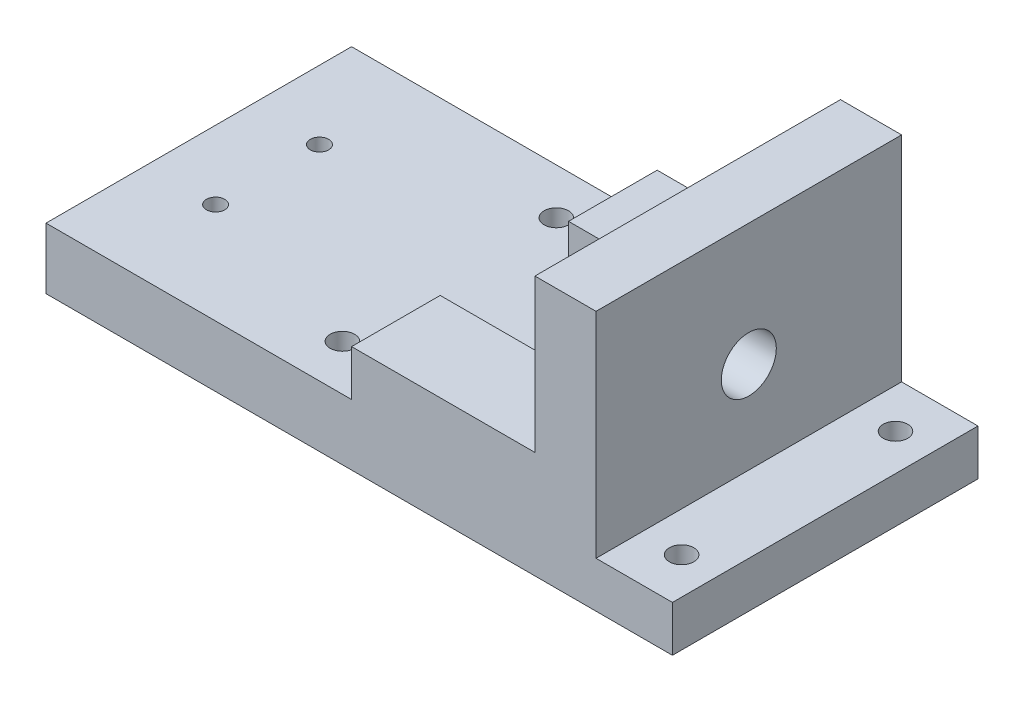
from build123d import *

# Parameters (mm, degrees)
BRACKET_BODY_DEPTH          = 50
BASE_HOLES_8_SET_A_SKETCH_R = 4
BASE_HOLES_8_SET_A_DEPTH    = 100
STEP_NOTCH_SKETCH_W         = 60
STEP_NOTCH_SKETCH_H         = 42
STEP_NOTCH_DEPTH            = 15
WEB_BORE_18_SKETCH_R        = 9
WEB_BORE_18_DEPTH           = 100
BASE_HOLES_8_SET_B_SKETCH_R = 4
BASE_HOLES_8_SET_B_DEPTH    = 100
BASE_HOLES_6_SKETCH_R       = 3
BASE_HOLES_6_DEPTH          = 100


with BuildPart() as part:
    # Bracket Profile Sketch → Bracket Body (new, symmetric)
    with BuildSketch(Plane.XY):
        Polygon((0, 0), (-102.5, 0), (-102.5, 20), (-2.5, 20), (-2.5, 35), (57.5, 35), (57.5, 85), (77.5, 85), (77.5, 15), (102.5, 15), (102.5, 0), align=None)
    extrude(amount=BRACKET_BODY_DEPTH, both=True)

    # Base Holes Ø8 Set A Sketch → Base Holes Ø8 Set A (cut)
    with BuildSketch(Plane(origin=(0, 15, 0), x_dir=(1, 0, 0), z_dir=(0, 1, 0))):
        with Locations(Location((90.5, 35, 0), (0, 0, 180))):
            Circle(BASE_HOLES_8_SET_A_SKETCH_R)
        with Locations(Location((90.5, -35, 0), (0, 0, 180))):
            Circle(BASE_HOLES_8_SET_A_SKETCH_R)
    extrude(amount=-BASE_HOLES_8_SET_A_DEPTH, mode=Mode.SUBTRACT)

    # Step Notch Sketch → Step Notch (cut)
    with BuildSketch(Plane(origin=(0, 35, 0), x_dir=(1, 0, 0), z_dir=(0, 1, 0))):
        with Locations((27.5, 0)):
            Rectangle(STEP_NOTCH_SKETCH_W, STEP_NOTCH_SKETCH_H)
    extrude(amount=-STEP_NOTCH_DEPTH, mode=Mode.SUBTRACT)

    # Web Bore Ø18 Sketch → Web Bore Ø18 (cut)
    with BuildSketch(Plane(origin=(77.5, 0, 0), x_dir=(0, 0, -1), z_dir=(1, 0, 0))):
        with Locations((0, 45)):
            Circle(WEB_BORE_18_SKETCH_R)
    extrude(amount=-WEB_BORE_18_DEPTH, mode=Mode.SUBTRACT)

    # Base Holes Ø8 Set B Sketch → Base Holes Ø8 Set B (cut)
    with BuildSketch(Plane(origin=(0, 20, 0), x_dir=(1, 0, 0), z_dir=(0, 1, 0))):
        with Locations(Location((-20.5, -35, 0), (0, 0, 180))):
            Circle(BASE_HOLES_8_SET_B_SKETCH_R)
        with Locations(Location((-20.5, 35, 0), (0, 0, 180))):
            Circle(BASE_HOLES_8_SET_B_SKETCH_R)
    extrude(amount=-BASE_HOLES_8_SET_B_DEPTH, mode=Mode.SUBTRACT)

    # Base Holes Ø6 Sketch → Base Holes Ø6 (cut)
    with BuildSketch(Plane(origin=(0, 20, 0), x_dir=(1, 0, 0), z_dir=(0, 1, 0))):
        with Locations(Location((-80, -17, 0), (0, 0, 180))):
            Circle(BASE_HOLES_6_SKETCH_R)
        with Locations(Location((-80, 17, 0), (0, 0, 180))):
            Circle(BASE_HOLES_6_SKETCH_R)
    extrude(amount=-BASE_HOLES_6_DEPTH, mode=Mode.SUBTRACT)


solid = part.part
